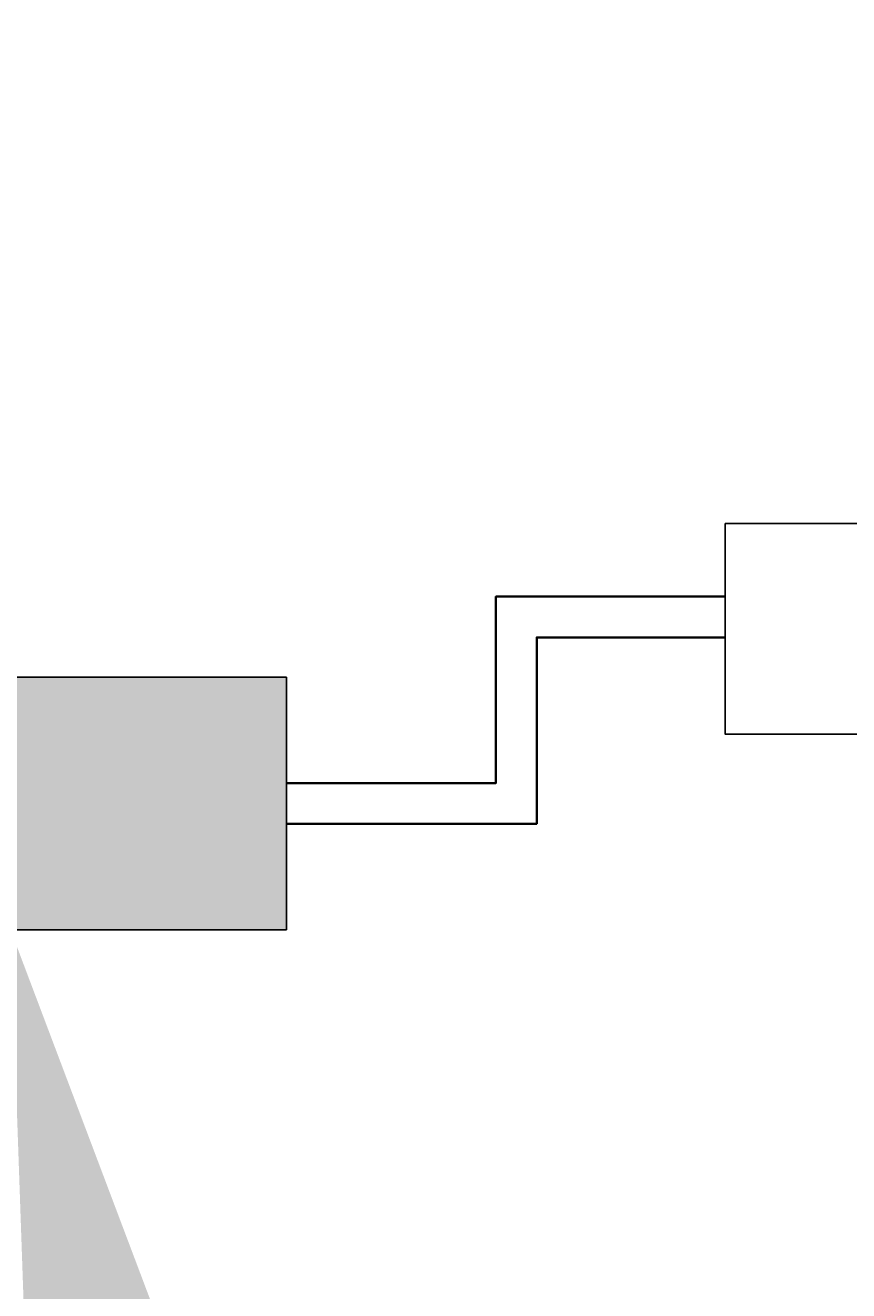
# Model space of a CAD drawing. Units: millimetres. Extents: x -22994 to 29398, y -19990 to 20176.
# Tile 14 of 135: x 58 to 79, y 21 to 52. Entities that reach past the tile are written whole.
import ezdxf
from ezdxf import colors
from ezdxf.entities.mleader import LeaderData, LeaderLine
from ezdxf.math import Vec2, Vec3

# ---------------------------------------------------------------- set-up
doc = ezdxf.new("R2010")
doc.units = ezdxf.units.MM
doc.header["$MEASUREMENT"] = 0
for name, color, linetype, lineweight in [('M-ANNO-TEXT', 7, 'Continuous', 25), ('M-DIMS', 2, 'Continuous', 18), ('M-EQPM', 7, 'Continuous', 25), ('M-EQPM-PATT', 7, 'Continuous', 18), ('M-PIPE', 7, 'Continuous', 35)]:
    doc.layers.add(name, color=color, linetype=linetype, lineweight=lineweight)
doc.styles.get("Standard").update_dxf_attribs({"font": 'arial.ttf'})
doc.dimstyles.get("Standard").update_dxf_attribs({"dimtxt": 0.18, "dimasz": 10000, "dimexe": 0.18, "dimexo": 0.0625, "dimgap": 0.09, "dimtad": 0, "dimtih": 1, "dimtoh": 1, "dimdec": 0, "dimzin": 0, "dimdsep": 46, "dimtxsty": 'Standard', "dimcen": 0.09, "dimadec": 0, "dimazin": 0, "dimtfac": 1, "dimtdec": 0, "dimtofl": 0, "dimtmove": 0, "dimatfit": 3, "dimfxl": 1, "dimtolj": 1, "dimtzin": 0, "dimlwd": 30, "dimarcsym": 0})

# ---------------------------------------------------------------- blocks, each defined once
blk = doc.blocks.new('*D2')
at = {"layer": 'Defpoints', "color": 0, "transparency": 16777216}
for p in [(6.677, 10.271), (290.852, 10.271), (290.852, -5.079)]:
    blk.add_point(p, dxfattribs=at)
at = {"layer": 'M-DIMS', "color": 0, "lineweight": -2, "transparency": 16777216}
for p, q in [((6.677, 10.209), (6.677, -5.259)), ((290.852, 10.209), (290.852, -5.259))]:
    blk.add_line(p, q, dxfattribs=at)
at = {"layer": 'M-DIMS', "color": 0, "lineweight": 30, "transparency": 16777216}
for p, q in [((-9993.323, -5.079), (-19993.323, -5.079)), ((10290.852, -5.079), (20290.852, -5.079))]:
    blk.add_line(p, q, dxfattribs=at)
at = {"layer": 'M-DIMS', "color": 0, "transparency": 16777216}
for points in [[(-9993.323, 1661.588), (-9993.323, -1671.745), (6.677, -5.079)], [(10290.852, 1661.588), (10290.852, -1671.745), (290.852, -5.079)]]:
    blk.add_solid(points, dxfattribs=at)
at = {"layer": 'M-DIMS', "color": 0, "transparency": 16777216, "insert": (148.765, -5.079), "char_height": 0.18, "attachment_point": 5}
blk.add_mtext('\\A1;284.2', dxfattribs=at)
blk = doc.blocks.new('*D3')
at = {"layer": 'Defpoints', "color": 0, "transparency": 16777216}
for p in [(110.265, 204.165), (110.265, 176.366), (95.833, 127.967)]:
    blk.add_point(p, dxfattribs=at)
at = {"layer": 'M-DIMS', "color": 0, "lineweight": 30, "transparency": 16777216}
for p, q in [((-9904.167, 204.165), (-19904.167, 204.165)), ((10110.265, 204.165), (20110.265, 204.165))]:
    blk.add_line(p, q, dxfattribs=at)
at = {"layer": 'M-DIMS', "color": 0, "lineweight": -2, "transparency": 16777216}
for p, q in [((95.833, 128.03), (95.833, 204.345)), ((110.265, 176.429), (110.265, 204.345))]:
    blk.add_line(p, q, dxfattribs=at)
at = {"layer": 'M-DIMS', "color": 0, "transparency": 16777216}
for points in [[(-9904.167, 1870.832), (-9904.167, -1462.501), (95.833, 204.165)], [(10110.265, 1870.832), (10110.265, -1462.501), (110.265, 204.165)]]:
    blk.add_solid(points, dxfattribs=at)
at = {"layer": 'M-DIMS', "color": 0, "transparency": 16777216, "insert": (103.049, 204.165), "char_height": 0.18, "attachment_point": 5}
blk.add_mtext('\\A1;14.432', dxfattribs=at)
blk = doc.blocks.new('*D4')
at = {"layer": 'Defpoints', "color": 0, "transparency": 16777216}
for p in [(116.265, 204.165), (110.265, 176.366), (116.265, 176.366)]:
    blk.add_point(p, dxfattribs=at)
at = {"layer": 'M-DIMS', "color": 0, "lineweight": 30, "transparency": 16777216}
for p, q in [((-9889.735, 204.165), (-19889.735, 204.165)), ((10116.265, 204.165), (20116.265, 204.165))]:
    blk.add_line(p, q, dxfattribs=at)
at = {"layer": 'M-DIMS', "color": 0, "lineweight": -2, "transparency": 16777216}
for p, q in [((110.265, 176.429), (110.265, 204.345)), ((116.265, 176.429), (116.265, 204.345))]:
    blk.add_line(p, q, dxfattribs=at)
at = {"layer": 'M-DIMS', "color": 0, "transparency": 16777216}
for points in [[(-9889.735, 1870.832), (-9889.735, -1462.501), (110.265, 204.165)], [(10116.265, 1870.832), (10116.265, -1462.501), (116.265, 204.165)]]:
    blk.add_solid(points, dxfattribs=at)
at = {"layer": 'M-DIMS', "color": 0, "transparency": 16777216, "insert": (113.265, 204.165), "char_height": 0.18, "attachment_point": 5}
blk.add_mtext('\\A1;6', dxfattribs=at)
blk = doc.blocks.new('*D5')
at = {"layer": 'Defpoints', "color": 0, "transparency": 16777216}
for p in [(181.265, 204.165), (116.265, 176.366), (181.265, 176.366)]:
    blk.add_point(p, dxfattribs=at)
at = {"layer": 'M-DIMS', "color": 0, "lineweight": 30, "transparency": 16777216}
for p, q in [((-9883.735, 204.165), (-19883.735, 204.165)), ((10181.265, 204.165), (20181.265, 204.165))]:
    blk.add_line(p, q, dxfattribs=at)
at = {"layer": 'M-DIMS', "color": 0, "lineweight": -2, "transparency": 16777216}
for p, q in [((116.265, 176.429), (116.265, 204.345)), ((181.265, 176.429), (181.265, 204.345))]:
    blk.add_line(p, q, dxfattribs=at)
at = {"layer": 'M-DIMS', "color": 0, "transparency": 16777216}
for points in [[(-9883.735, 1870.832), (-9883.735, -1462.501), (116.265, 204.165)], [(10181.265, 1870.832), (10181.265, -1462.501), (181.265, 204.165)]]:
    blk.add_solid(points, dxfattribs=at)
at = {"layer": 'M-DIMS', "color": 0, "transparency": 16777216, "insert": (148.765, 204.165), "char_height": 0.18, "attachment_point": 5}
blk.add_mtext('\\A1;65', dxfattribs=at)
blk = doc.blocks.new('*D6')
at = {"layer": 'Defpoints', "color": 0, "transparency": 16777216}
for p in [(187.265, 204.165), (181.265, 176.366), (187.265, 176.366)]:
    blk.add_point(p, dxfattribs=at)
at = {"layer": 'M-DIMS', "color": 0, "lineweight": 30, "transparency": 16777216}
for p, q in [((-9818.735, 204.165), (-19818.735, 204.165)), ((10187.265, 204.165), (20187.265, 204.165))]:
    blk.add_line(p, q, dxfattribs=at)
at = {"layer": 'M-DIMS', "color": 0, "lineweight": -2, "transparency": 16777216}
for p, q in [((181.265, 176.429), (181.265, 204.345)), ((187.265, 176.429), (187.265, 204.345))]:
    blk.add_line(p, q, dxfattribs=at)
at = {"layer": 'M-DIMS', "color": 0, "transparency": 16777216}
for points in [[(-9818.735, 1870.832), (-9818.735, -1462.501), (181.265, 204.165)], [(10187.265, 1870.832), (10187.265, -1462.501), (187.265, 204.165)]]:
    blk.add_solid(points, dxfattribs=at)
at = {"layer": 'M-DIMS', "color": 0, "transparency": 16777216, "insert": (184.265, 204.165), "char_height": 0.18, "attachment_point": 5}
blk.add_mtext('\\A1;6', dxfattribs=at)
blk = doc.blocks.new('*D7')
at = {"layer": 'Defpoints', "color": 0, "transparency": 16777216}
for p in [(201.697, 204.165), (187.265, 176.366), (201.697, 127.967)]:
    blk.add_point(p, dxfattribs=at)
at = {"layer": 'M-DIMS', "color": 0, "lineweight": 30, "transparency": 16777216}
for p, q in [((-9812.735, 204.165), (-19812.735, 204.165)), ((10201.697, 204.165), (20201.697, 204.165))]:
    blk.add_line(p, q, dxfattribs=at)
at = {"layer": 'M-DIMS', "color": 0, "lineweight": -2, "transparency": 16777216}
for p, q in [((187.265, 176.429), (187.265, 204.345)), ((201.697, 128.03), (201.697, 204.345))]:
    blk.add_line(p, q, dxfattribs=at)
at = {"layer": 'M-DIMS', "color": 0, "transparency": 16777216}
for points in [[(-9812.735, 1870.832), (-9812.735, -1462.501), (187.265, 204.165)], [(10201.697, 1870.832), (10201.697, -1462.501), (201.697, 204.165)]]:
    blk.add_solid(points, dxfattribs=at)
at = {"layer": 'M-DIMS', "color": 0, "transparency": 16777216, "insert": (194.481, 204.165), "char_height": 0.18, "attachment_point": 5}
blk.add_mtext('\\A1;14.432', dxfattribs=at)
blk = doc.blocks.new('*D8')
at = {"layer": 'Defpoints', "color": 0, "transparency": 16777216}
for p in [(227.648, 204.165), (227.648, 146.73), (201.697, 127.967)]:
    blk.add_point(p, dxfattribs=at)
at = {"layer": 'M-DIMS', "color": 0, "lineweight": 30, "transparency": 16777216}
for p, q in [((-9798.303, 204.165), (-19798.303, 204.165)), ((10227.648, 204.165), (20227.648, 204.165))]:
    blk.add_line(p, q, dxfattribs=at)
at = {"layer": 'M-DIMS', "color": 0, "lineweight": -2, "transparency": 16777216}
for p, q in [((201.697, 128.03), (201.697, 204.345)), ((227.648, 146.792), (227.648, 204.345))]:
    blk.add_line(p, q, dxfattribs=at)
at = {"layer": 'M-DIMS', "color": 0, "transparency": 16777216}
for points in [[(-9798.303, 1870.832), (-9798.303, -1462.501), (201.697, 204.165)], [(10227.648, 1870.832), (10227.648, -1462.501), (227.648, 204.165)]]:
    blk.add_solid(points, dxfattribs=at)
at = {"layer": 'M-DIMS', "color": 0, "transparency": 16777216, "insert": (214.673, 204.165), "char_height": 0.18, "attachment_point": 5}
blk.add_mtext('\\A1;25.95', dxfattribs=at)
blk = doc.blocks.new('*D9')
at = {"layer": 'Defpoints', "color": 0, "transparency": 16777216}
for p in [(187.265, 176.366), (306.202, 176.366), (290.852, 10.271)]:
    blk.add_point(p, dxfattribs=at)
at = {"layer": 'M-DIMS', "color": 0, "lineweight": 30, "transparency": 16777216}
for p, q in [((306.202, 10176.366), (306.202, 20176.366)), ((306.202, -9989.729), (306.202, -19989.729))]:
    blk.add_line(p, q, dxfattribs=at)
at = {"layer": 'M-DIMS', "color": 0, "lineweight": -2, "transparency": 16777216}
for p, q in [((187.327, 176.366), (306.382, 176.366)), ((290.915, 10.271), (306.382, 10.271))]:
    blk.add_line(p, q, dxfattribs=at)
at = {"layer": 'M-DIMS', "color": 0, "transparency": 16777216}
for points in [[(-1360.465, 10176.366), (1972.869, 10176.366), (306.202, 176.366)], [(-1360.465, -9989.729), (1972.869, -9989.729), (306.202, 10.271)]]:
    blk.add_solid(points, dxfattribs=at)
at = {"layer": 'M-DIMS', "color": 0, "transparency": 16777216, "insert": (306.202, 93.319), "char_height": 0.18, "attachment_point": 5}
blk.add_mtext('\\A1;166.1', dxfattribs=at)
blk = doc.blocks.new('*D10')
at = {"layer": 'Defpoints', "color": 0, "transparency": 16777216}
for p in [(125.65, 136.071), (133.346, 136.071), (133.346, -5.079)]:
    blk.add_point(p, dxfattribs=at)
at = {"layer": 'M-DIMS', "color": 0, "lineweight": -2, "transparency": 16777216}
for p, q in [((125.65, 136.009), (125.65, -5.259)), ((133.346, 136.009), (133.346, -5.259))]:
    blk.add_line(p, q, dxfattribs=at)
at = {"layer": 'M-DIMS', "color": 0, "lineweight": 30, "transparency": 16777216}
for p, q in [((-9874.35, -5.079), (-19874.35, -5.079)), ((10133.346, -5.079), (20133.346, -5.079))]:
    blk.add_line(p, q, dxfattribs=at)
at = {"layer": 'M-DIMS', "color": 0, "transparency": 16777216}
for points in [[(-9874.35, 1661.588), (-9874.35, -1671.745), (125.65, -5.079)], [(10133.346, 1661.588), (10133.346, -1671.745), (133.346, -5.079)]]:
    blk.add_solid(points, dxfattribs=at)
at = {"layer": 'M-DIMS', "color": 0, "transparency": 16777216, "insert": (129.498, -5.079), "char_height": 0.18, "attachment_point": 5}
blk.add_mtext('\\A1;7.696', dxfattribs=at)
blk = doc.blocks.new('*D11')
at = {"layer": 'Defpoints', "color": 0, "transparency": 16777216}
for p in [(133.346, 136.071), (135.65, 136.071), (135.65, -5.079)]:
    blk.add_point(p, dxfattribs=at)
at = {"layer": 'M-DIMS', "color": 0, "lineweight": -2, "transparency": 16777216}
for p, q in [((133.346, 136.009), (133.346, -5.259)), ((135.65, 136.009), (135.65, -5.259))]:
    blk.add_line(p, q, dxfattribs=at)
at = {"layer": 'M-DIMS', "color": 0, "lineweight": 30, "transparency": 16777216}
for p, q in [((-9866.654, -5.079), (-19866.654, -5.079)), ((10135.65, -5.079), (20135.65, -5.079))]:
    blk.add_line(p, q, dxfattribs=at)
at = {"layer": 'M-DIMS', "color": 0, "transparency": 16777216}
for points in [[(-9866.654, 1661.588), (-9866.654, -1671.745), (133.346, -5.079)], [(10135.65, 1661.588), (10135.65, -1671.745), (135.65, -5.079)]]:
    blk.add_solid(points, dxfattribs=at)
at = {"layer": 'M-DIMS', "color": 0, "transparency": 16777216, "insert": (134.498, -5.079), "char_height": 0.18, "attachment_point": 5}
blk.add_mtext('\\A1;2.304', dxfattribs=at)
blk = doc.blocks.new('*D12')
at = {"layer": 'Defpoints', "color": 0, "transparency": 16777216}
for p in [(135.65, 136.071), (145.65, 136.071), (145.65, -5.079)]:
    blk.add_point(p, dxfattribs=at)
at = {"layer": 'M-DIMS', "color": 0, "lineweight": -2, "transparency": 16777216}
for p, q in [((135.65, 136.009), (135.65, -5.259)), ((145.65, 136.009), (145.65, -5.259))]:
    blk.add_line(p, q, dxfattribs=at)
at = {"layer": 'M-DIMS', "color": 0, "lineweight": 30, "transparency": 16777216}
for p, q in [((-9864.35, -5.079), (-19864.35, -5.079)), ((10145.65, -5.079), (20145.65, -5.079))]:
    blk.add_line(p, q, dxfattribs=at)
at = {"layer": 'M-DIMS', "color": 0, "transparency": 16777216}
for points in [[(-9864.35, 1661.588), (-9864.35, -1671.745), (135.65, -5.079)], [(10145.65, 1661.588), (10145.65, -1671.745), (145.65, -5.079)]]:
    blk.add_solid(points, dxfattribs=at)
at = {"layer": 'M-DIMS', "color": 0, "transparency": 16777216, "insert": (140.65, -5.079), "char_height": 0.18, "attachment_point": 5}
blk.add_mtext('\\A1;10', dxfattribs=at)
blk = doc.blocks.new('*D13')
at = {"layer": 'Defpoints', "color": 0, "transparency": 16777216}
for p in [(145.65, 136.071), (155.65, 136.071), (155.65, -5.079)]:
    blk.add_point(p, dxfattribs=at)
at = {"layer": 'M-DIMS', "color": 0, "lineweight": -2, "transparency": 16777216}
for p, q in [((145.65, 136.009), (145.65, -5.259)), ((155.65, 136.009), (155.65, -5.259))]:
    blk.add_line(p, q, dxfattribs=at)
at = {"layer": 'M-DIMS', "color": 0, "lineweight": 30, "transparency": 16777216}
for p, q in [((-9854.35, -5.079), (-19854.35, -5.079)), ((10155.65, -5.079), (20155.65, -5.079))]:
    blk.add_line(p, q, dxfattribs=at)
at = {"layer": 'M-DIMS', "color": 0, "transparency": 16777216}
for points in [[(-9854.35, 1661.588), (-9854.35, -1671.745), (145.65, -5.079)], [(10155.65, 1661.588), (10155.65, -1671.745), (155.65, -5.079)]]:
    blk.add_solid(points, dxfattribs=at)
at = {"layer": 'M-DIMS', "color": 0, "transparency": 16777216, "insert": (150.65, -5.079), "char_height": 0.18, "attachment_point": 5}
blk.add_mtext('\\A1;10', dxfattribs=at)
blk = doc.blocks.new('*D14')
at = {"layer": 'Defpoints', "color": 0, "transparency": 16777216}
for p in [(155.65, 136.071), (165.65, 136.071), (165.65, -5.079)]:
    blk.add_point(p, dxfattribs=at)
at = {"layer": 'M-DIMS', "color": 0, "lineweight": -2, "transparency": 16777216}
for p, q in [((155.65, 136.009), (155.65, -5.259)), ((165.65, 136.009), (165.65, -5.259))]:
    blk.add_line(p, q, dxfattribs=at)
at = {"layer": 'M-DIMS', "color": 0, "lineweight": 30, "transparency": 16777216}
for p, q in [((-9844.35, -5.079), (-19844.35, -5.079)), ((10165.65, -5.079), (20165.65, -5.079))]:
    blk.add_line(p, q, dxfattribs=at)
at = {"layer": 'M-DIMS', "color": 0, "transparency": 16777216}
for points in [[(-9844.35, 1661.588), (-9844.35, -1671.745), (155.65, -5.079)], [(10165.65, 1661.588), (10165.65, -1671.745), (165.65, -5.079)]]:
    blk.add_solid(points, dxfattribs=at)
at = {"layer": 'M-DIMS', "color": 0, "transparency": 16777216, "insert": (160.65, -5.079), "char_height": 0.18, "attachment_point": 5}
blk.add_mtext('\\A1;10', dxfattribs=at)
blk = doc.blocks.new('*D15')
at = {"layer": 'Defpoints', "color": 0, "transparency": 16777216}
for p in [(173.346, 154.788), (173.346, 136.071), (306.202, 136.071)]:
    blk.add_point(p, dxfattribs=at)
at = {"layer": 'M-DIMS', "color": 0, "lineweight": 30, "transparency": 16777216}
for p, q in [((306.202, 10154.788), (306.202, 20154.788)), ((306.202, -9863.929), (306.202, -19863.929))]:
    blk.add_line(p, q, dxfattribs=at)
at = {"layer": 'M-DIMS', "color": 0, "lineweight": -2, "transparency": 16777216}
for p, q in [((173.408, 154.788), (306.382, 154.788)), ((173.408, 136.071), (306.382, 136.071))]:
    blk.add_line(p, q, dxfattribs=at)
at = {"layer": 'M-DIMS', "color": 0, "transparency": 16777216}
for points in [[(-1360.465, 10154.788), (1972.869, 10154.788), (306.202, 154.788)], [(-1360.465, -9863.929), (1972.869, -9863.929), (306.202, 136.071)]]:
    blk.add_solid(points, dxfattribs=at)
at = {"layer": 'M-DIMS', "color": 0, "transparency": 16777216, "insert": (306.202, 145.43), "char_height": 0.18, "attachment_point": 5}
blk.add_mtext('\\A1;18.717', dxfattribs=at)
blk = doc.blocks.new('*D16')
at = {"layer": 'Defpoints', "color": 0, "transparency": 16777216}
for p in [(120.17, 204.165), (110.466, 48.035), (120.17, 48.035)]:
    blk.add_point(p, dxfattribs=at)
at = {"layer": 'M-DIMS', "color": 0, "lineweight": 30, "transparency": 16777216}
for p, q in [((-9889.534, 204.165), (-19889.534, 204.165)), ((10120.17, 204.165), (20120.17, 204.165))]:
    blk.add_line(p, q, dxfattribs=at)
at = {"layer": 'M-DIMS', "color": 0, "lineweight": -2, "transparency": 16777216}
for p, q in [((110.466, 48.097), (110.466, 204.345)), ((120.17, 48.097), (120.17, 204.345))]:
    blk.add_line(p, q, dxfattribs=at)
at = {"layer": 'M-DIMS', "color": 0, "transparency": 16777216}
for points in [[(-9889.534, 1870.832), (-9889.534, -1462.501), (110.466, 204.165)], [(10120.17, 1870.832), (10120.17, -1462.501), (120.17, 204.165)]]:
    blk.add_solid(points, dxfattribs=at)
at = {"layer": 'M-DIMS', "color": 0, "transparency": 16777216, "insert": (115.318, 204.165), "char_height": 0.18, "attachment_point": 5}
blk.add_mtext('\\A1;9.704', dxfattribs=at)
blk = doc.blocks.new('*D17')
at = {"layer": 'Defpoints', "color": 0, "transparency": 16777216}
for p in [(126.17, 204.165), (120.17, 48.035), (126.17, 48.035)]:
    blk.add_point(p, dxfattribs=at)
at = {"layer": 'M-DIMS', "color": 0, "lineweight": 30, "transparency": 16777216}
for p, q in [((-9879.83, 204.165), (-19879.83, 204.165)), ((10126.17, 204.165), (20126.17, 204.165))]:
    blk.add_line(p, q, dxfattribs=at)
at = {"layer": 'M-DIMS', "color": 0, "lineweight": -2, "transparency": 16777216}
for p, q in [((120.17, 48.097), (120.17, 204.345)), ((126.17, 48.097), (126.17, 204.345))]:
    blk.add_line(p, q, dxfattribs=at)
at = {"layer": 'M-DIMS', "color": 0, "transparency": 16777216}
for points in [[(-9879.83, 1870.832), (-9879.83, -1462.501), (120.17, 204.165)], [(10126.17, 1870.832), (10126.17, -1462.501), (126.17, 204.165)]]:
    blk.add_solid(points, dxfattribs=at)
at = {"layer": 'M-DIMS', "color": 0, "transparency": 16777216, "insert": (123.17, 204.165), "char_height": 0.18, "attachment_point": 5}
blk.add_mtext('\\A1;6', dxfattribs=at)
blk = doc.blocks.new('*D18')
at = {"layer": 'Defpoints', "color": 0, "transparency": 16777216}
for p in [(132.17, 204.165), (126.17, 48.035), (132.17, 48.035)]:
    blk.add_point(p, dxfattribs=at)
at = {"layer": 'M-DIMS', "color": 0, "lineweight": 30, "transparency": 16777216}
for p, q in [((-9873.83, 204.165), (-19873.83, 204.165)), ((10132.17, 204.165), (20132.17, 204.165))]:
    blk.add_line(p, q, dxfattribs=at)
at = {"layer": 'M-DIMS', "color": 0, "lineweight": -2, "transparency": 16777216}
for p, q in [((126.17, 48.097), (126.17, 204.345)), ((132.17, 48.097), (132.17, 204.345))]:
    blk.add_line(p, q, dxfattribs=at)
at = {"layer": 'M-DIMS', "color": 0, "transparency": 16777216}
for points in [[(-9873.83, 1870.832), (-9873.83, -1462.501), (126.17, 204.165)], [(10132.17, 1870.832), (10132.17, -1462.501), (132.17, 204.165)]]:
    blk.add_solid(points, dxfattribs=at)
at = {"layer": 'M-DIMS', "color": 0, "transparency": 16777216, "insert": (129.17, 204.165), "char_height": 0.18, "attachment_point": 5}
blk.add_mtext('\\A1;6', dxfattribs=at)
blk = doc.blocks.new('*D19')
at = {"layer": 'Defpoints', "color": 0, "transparency": 16777216}
for p in [(138.17, 204.165), (132.17, 48.035), (138.17, 48.035)]:
    blk.add_point(p, dxfattribs=at)
at = {"layer": 'M-DIMS', "color": 0, "lineweight": 30, "transparency": 16777216}
for p, q in [((-9867.83, 204.165), (-19867.83, 204.165)), ((10138.17, 204.165), (20138.17, 204.165))]:
    blk.add_line(p, q, dxfattribs=at)
at = {"layer": 'M-DIMS', "color": 0, "lineweight": -2, "transparency": 16777216}
for p, q in [((132.17, 48.097), (132.17, 204.345)), ((138.17, 48.097), (138.17, 204.345))]:
    blk.add_line(p, q, dxfattribs=at)
at = {"layer": 'M-DIMS', "color": 0, "transparency": 16777216}
for points in [[(-9867.83, 1870.832), (-9867.83, -1462.501), (132.17, 204.165)], [(10138.17, 1870.832), (10138.17, -1462.501), (138.17, 204.165)]]:
    blk.add_solid(points, dxfattribs=at)
at = {"layer": 'M-DIMS', "color": 0, "transparency": 16777216, "insert": (135.17, 204.165), "char_height": 0.18, "attachment_point": 5}
blk.add_mtext('\\A1;6', dxfattribs=at)
blk = doc.blocks.new('*D20')
at = {"layer": 'Defpoints', "color": 0, "transparency": 16777216}
for p in [(144.17, 204.165), (138.17, 48.035), (144.17, 48.035)]:
    blk.add_point(p, dxfattribs=at)
at = {"layer": 'M-DIMS', "color": 0, "lineweight": 30, "transparency": 16777216}
for p, q in [((-9861.83, 204.165), (-19861.83, 204.165)), ((10144.17, 204.165), (20144.17, 204.165))]:
    blk.add_line(p, q, dxfattribs=at)
at = {"layer": 'M-DIMS', "color": 0, "lineweight": -2, "transparency": 16777216}
for p, q in [((138.17, 48.097), (138.17, 204.345)), ((144.17, 48.097), (144.17, 204.345))]:
    blk.add_line(p, q, dxfattribs=at)
at = {"layer": 'M-DIMS', "color": 0, "transparency": 16777216}
for points in [[(-9861.83, 1870.832), (-9861.83, -1462.501), (138.17, 204.165)], [(10144.17, 1870.832), (10144.17, -1462.501), (144.17, 204.165)]]:
    blk.add_solid(points, dxfattribs=at)
at = {"layer": 'M-DIMS', "color": 0, "transparency": 16777216, "insert": (141.17, 204.165), "char_height": 0.18, "attachment_point": 5}
blk.add_mtext('\\A1;6', dxfattribs=at)
blk = doc.blocks.new('*D21')
at = {"layer": 'Defpoints', "color": 0, "transparency": 16777216}
for p in [(149.116, 204.165), (144.17, 48.035), (149.116, 48.035)]:
    blk.add_point(p, dxfattribs=at)
at = {"layer": 'M-DIMS', "color": 0, "lineweight": 30, "transparency": 16777216}
for p, q in [((-9855.83, 204.165), (-19855.83, 204.165)), ((10149.116, 204.165), (20149.116, 204.165))]:
    blk.add_line(p, q, dxfattribs=at)
at = {"layer": 'M-DIMS', "color": 0, "lineweight": -2, "transparency": 16777216}
for p, q in [((144.17, 48.097), (144.17, 204.345)), ((149.116, 48.097), (149.116, 204.345))]:
    blk.add_line(p, q, dxfattribs=at)
at = {"layer": 'M-DIMS', "color": 0, "transparency": 16777216}
for points in [[(-9855.83, 1870.832), (-9855.83, -1462.501), (144.17, 204.165)], [(10149.116, 1870.832), (10149.116, -1462.501), (149.116, 204.165)]]:
    blk.add_solid(points, dxfattribs=at)
at = {"layer": 'M-DIMS', "color": 0, "transparency": 16777216, "insert": (146.643, 204.165), "char_height": 0.18, "attachment_point": 5}
blk.add_mtext('\\A1;4.945', dxfattribs=at)
blk = doc.blocks.new('*D22')
at = {"layer": 'Defpoints', "color": 0, "transparency": 16777216}
for p in [(149.116, 30.99), (155.116, 30.99), (155.116, -5.079)]:
    blk.add_point(p, dxfattribs=at)
at = {"layer": 'M-DIMS', "color": 0, "lineweight": -2, "transparency": 16777216}
for p, q in [((149.116, 30.927), (149.116, -5.259)), ((155.116, 30.927), (155.116, -5.259))]:
    blk.add_line(p, q, dxfattribs=at)
at = {"layer": 'M-DIMS', "color": 0, "lineweight": 30, "transparency": 16777216}
for p, q in [((-9850.884, -5.079), (-19850.884, -5.079)), ((10155.116, -5.079), (20155.116, -5.079))]:
    blk.add_line(p, q, dxfattribs=at)
at = {"layer": 'M-DIMS', "color": 0, "transparency": 16777216}
for points in [[(-9850.884, 1661.588), (-9850.884, -1671.745), (149.116, -5.079)], [(10155.116, 1661.588), (10155.116, -1671.745), (155.116, -5.079)]]:
    blk.add_solid(points, dxfattribs=at)
at = {"layer": 'M-DIMS', "color": 0, "transparency": 16777216, "insert": (152.116, -5.079), "char_height": 0.18, "attachment_point": 5}
blk.add_mtext('\\A1;6', dxfattribs=at)
blk = doc.blocks.new('*D23')
at = {"layer": 'Defpoints', "color": 0, "transparency": 16777216}
for p in [(155.116, 30.99), (161.116, 30.99), (161.116, -5.079)]:
    blk.add_point(p, dxfattribs=at)
at = {"layer": 'M-DIMS', "color": 0, "lineweight": -2, "transparency": 16777216}
for p, q in [((155.116, 30.927), (155.116, -5.259)), ((161.116, 30.927), (161.116, -5.259))]:
    blk.add_line(p, q, dxfattribs=at)
at = {"layer": 'M-DIMS', "color": 0, "lineweight": 30, "transparency": 16777216}
for p, q in [((-9844.884, -5.079), (-19844.884, -5.079)), ((10161.116, -5.079), (20161.116, -5.079))]:
    blk.add_line(p, q, dxfattribs=at)
at = {"layer": 'M-DIMS', "color": 0, "transparency": 16777216}
for points in [[(-9844.884, 1661.588), (-9844.884, -1671.745), (155.116, -5.079)], [(10161.116, 1661.588), (10161.116, -1671.745), (161.116, -5.079)]]:
    blk.add_solid(points, dxfattribs=at)
at = {"layer": 'M-DIMS', "color": 0, "transparency": 16777216, "insert": (158.116, -5.079), "char_height": 0.18, "attachment_point": 5}
blk.add_mtext('\\A1;6', dxfattribs=at)
blk = doc.blocks.new('*D24')
at = {"layer": 'Defpoints', "color": 0, "transparency": 16777216}
for p in [(161.116, 30.99), (166.439, 30.99), (166.439, -5.079)]:
    blk.add_point(p, dxfattribs=at)
at = {"layer": 'M-DIMS', "color": 0, "lineweight": -2, "transparency": 16777216}
for p, q in [((161.116, 30.927), (161.116, -5.259)), ((166.439, 30.927), (166.439, -5.259))]:
    blk.add_line(p, q, dxfattribs=at)
at = {"layer": 'M-DIMS', "color": 0, "lineweight": 30, "transparency": 16777216}
for p, q in [((-9838.884, -5.079), (-19838.884, -5.079)), ((10166.439, -5.079), (20166.439, -5.079))]:
    blk.add_line(p, q, dxfattribs=at)
at = {"layer": 'M-DIMS', "color": 0, "transparency": 16777216}
for points in [[(-9838.884, 1661.588), (-9838.884, -1671.745), (161.116, -5.079)], [(10166.439, 1661.588), (10166.439, -1671.745), (166.439, -5.079)]]:
    blk.add_solid(points, dxfattribs=at)
at = {"layer": 'M-DIMS', "color": 0, "transparency": 16777216, "insert": (163.777, -5.079), "char_height": 0.18, "attachment_point": 5}
blk.add_mtext('\\A1;5.323', dxfattribs=at)
blk = doc.blocks.new('*D25')
at = {"layer": 'Defpoints', "color": 0, "transparency": 16777216}
for p in [(166.439, 30.99), (172.439, 30.99), (172.439, -5.079)]:
    blk.add_point(p, dxfattribs=at)
at = {"layer": 'M-DIMS', "color": 0, "lineweight": -2, "transparency": 16777216}
for p, q in [((166.439, 30.927), (166.439, -5.259)), ((172.439, 30.927), (172.439, -5.259))]:
    blk.add_line(p, q, dxfattribs=at)
at = {"layer": 'M-DIMS', "color": 0, "lineweight": 30, "transparency": 16777216}
for p, q in [((-9833.561, -5.079), (-19833.561, -5.079)), ((10172.439, -5.079), (20172.439, -5.079))]:
    blk.add_line(p, q, dxfattribs=at)
at = {"layer": 'M-DIMS', "color": 0, "transparency": 16777216}
for points in [[(-9833.561, 1661.588), (-9833.561, -1671.745), (166.439, -5.079)], [(10172.439, 1661.588), (10172.439, -1671.745), (172.439, -5.079)]]:
    blk.add_solid(points, dxfattribs=at)
at = {"layer": 'M-DIMS', "color": 0, "transparency": 16777216, "insert": (169.439, -5.079), "char_height": 0.18, "attachment_point": 5}
blk.add_mtext('\\A1;6', dxfattribs=at)
blk = doc.blocks.new('*D26')
at = {"layer": 'Defpoints', "color": 0, "transparency": 16777216}
for p in [(172.439, 30.99), (178.439, 30.99), (178.439, -5.079)]:
    blk.add_point(p, dxfattribs=at)
at = {"layer": 'M-DIMS', "color": 0, "lineweight": -2, "transparency": 16777216}
for p, q in [((172.439, 30.927), (172.439, -5.259)), ((178.439, 30.927), (178.439, -5.259))]:
    blk.add_line(p, q, dxfattribs=at)
at = {"layer": 'M-DIMS', "color": 0, "lineweight": 30, "transparency": 16777216}
for p, q in [((-9827.561, -5.079), (-19827.561, -5.079)), ((10178.439, -5.079), (20178.439, -5.079))]:
    blk.add_line(p, q, dxfattribs=at)
at = {"layer": 'M-DIMS', "color": 0, "transparency": 16777216}
for points in [[(-9827.561, 1661.588), (-9827.561, -1671.745), (172.439, -5.079)], [(10178.439, 1661.588), (10178.439, -1671.745), (178.439, -5.079)]]:
    blk.add_solid(points, dxfattribs=at)
at = {"layer": 'M-DIMS', "color": 0, "transparency": 16777216, "insert": (175.439, -5.079), "char_height": 0.18, "attachment_point": 5}
blk.add_mtext('\\A1;6', dxfattribs=at)
blk = doc.blocks.new('*D27')
at = {"layer": 'Defpoints', "color": 0, "transparency": 16777216}
for p in [(178.439, 30.99), (188.117, 30.99), (188.117, -5.079)]:
    blk.add_point(p, dxfattribs=at)
at = {"layer": 'M-DIMS', "color": 0, "lineweight": -2, "transparency": 16777216}
for p, q in [((178.439, 30.927), (178.439, -5.259)), ((188.117, 30.927), (188.117, -5.259))]:
    blk.add_line(p, q, dxfattribs=at)
at = {"layer": 'M-DIMS', "color": 0, "lineweight": 30, "transparency": 16777216}
for p, q in [((-9821.561, -5.079), (-19821.561, -5.079)), ((10188.117, -5.079), (20188.117, -5.079))]:
    blk.add_line(p, q, dxfattribs=at)
at = {"layer": 'M-DIMS', "color": 0, "transparency": 16777216}
for points in [[(-9821.561, 1661.588), (-9821.561, -1671.745), (178.439, -5.079)], [(10188.117, 1661.588), (10188.117, -1671.745), (188.117, -5.079)]]:
    blk.add_solid(points, dxfattribs=at)
at = {"layer": 'M-DIMS', "color": 0, "transparency": 16777216, "insert": (183.278, -5.079), "char_height": 0.18, "attachment_point": 5}
blk.add_mtext('\\A1;9.679', dxfattribs=at)
blk = doc.blocks.new('*D28')
at = {"layer": 'Defpoints', "color": 0, "transparency": 16777216}
for p in [(188.117, 48.035), (306.202, 48.035), (188.117, 30.99)]:
    blk.add_point(p, dxfattribs=at)
at = {"layer": 'M-DIMS', "color": 0, "lineweight": 30, "transparency": 16777216}
for p, q in [((306.202, 10048.035), (306.202, 20048.035)), ((306.202, -9969.01), (306.202, -19969.01))]:
    blk.add_line(p, q, dxfattribs=at)
at = {"layer": 'M-DIMS', "color": 0, "lineweight": -2, "transparency": 16777216}
for p, q in [((188.18, 48.035), (306.382, 48.035)), ((188.18, 30.99), (306.382, 30.99))]:
    blk.add_line(p, q, dxfattribs=at)
at = {"layer": 'M-DIMS', "color": 0, "transparency": 16777216}
for points in [[(-1360.465, 10048.035), (1972.869, 10048.035), (306.202, 48.035)], [(-1360.465, -9969.01), (1972.869, -9969.01), (306.202, 30.99)]]:
    blk.add_solid(points, dxfattribs=at)
at = {"layer": 'M-DIMS', "color": 0, "transparency": 16777216, "insert": (306.202, 39.512), "char_height": 0.18, "attachment_point": 5}
blk.add_mtext('\\A1;17.045', dxfattribs=at)
blk = doc.blocks.new('*D29')
at = {"layer": 'Defpoints', "color": 0, "transparency": 16777216}
for p in [(36.801, 80.045), (64.03, 80.045)]:
    blk.add_point(p, dxfattribs=at)
at = {"layer": 'M-DIMS', "color": 0, "lineweight": -2, "transparency": 16777216}
for p, q in [((50.325, 80.045), (50.505, 80.045)), ((50.415, 79.955), (50.415, 80.135))]:
    blk.add_line(p, q, dxfattribs=at)
at = {"layer": 'M-DIMS', "color": 0, "lineweight": 30, "transparency": 16777216}
blk.add_line((20064.03, 80.03), (10064.03, 80.038), dxfattribs=at)
at = {"layer": 'M-DIMS', "color": 0, "transparency": 16777216}
blk.add_solid([(10064.031, 1746.704), (10064.028, -1586.629), (64.03, 80.045)], dxfattribs=at)
at = {"layer": 'M-DIMS', "color": 0, "transparency": 16777216, "insert": (20064.521, 80.03), "char_height": 0.18, "attachment_point": 5}
blk.add_mtext('\\A1;∅27.23', dxfattribs=at)
blk = doc.blocks.new('*D36')
at = {"layer": 'Defpoints', "color": 0, "transparency": 16777216}
for p in [(46.39, 31.303), (46.387, 26.593)]:
    blk.add_point(p, dxfattribs=at)
at = {"layer": 'M-DIMS', "color": 0, "lineweight": 30, "transparency": 16777216}
for p, q in [((57.15, 20031.301), (51.77, 10031.302)), ((10057.15, 20031.301), (57.15, 20031.301))]:
    blk.add_line(p, q, dxfattribs=at)
at = {"layer": 'M-DIMS', "color": 0, "lineweight": -2, "transparency": 16777216}
for p, q in [((46.299, 28.948), (46.479, 28.948)), ((46.389, 28.858), (46.389, 29.038))]:
    blk.add_line(p, q, dxfattribs=at)
at = {"layer": 'M-DIMS', "color": 0, "transparency": 16777216}
blk.add_solid([(-1614.896, 10032.199), (1718.436, 10030.405), (46.39, 31.303)], dxfattribs=at)
at = {"layer": 'M-DIMS', "color": 0, "transparency": 16777216, "insert": (10057.554, 20031.301), "char_height": 0.18, "attachment_point": 5}
blk.add_mtext('\\A1;∅4.71', dxfattribs=at)
blk = doc.blocks.new('*D37')
at = {"layer": 'Defpoints', "color": 0, "transparency": 16777216}
for p in [(54.834, 118.615), (59.494, 118.614)]:
    blk.add_point(p, dxfattribs=at)
at = {"layer": 'M-DIMS', "color": 0, "lineweight": -2, "transparency": 16777216}
for p, q in [((57.074, 118.614), (57.254, 118.614)), ((57.164, 118.524), (57.164, 118.704))]:
    blk.add_line(p, q, dxfattribs=at)
at = {"layer": 'M-DIMS', "color": 0, "lineweight": 30, "transparency": 16777216}
blk.add_line((20059.493, 116.253), (10059.494, 117.434), dxfattribs=at)
at = {"layer": 'M-DIMS', "color": 0, "transparency": 16777216}
blk.add_solid([(10059.69, 1784.1), (10059.297, -1549.233), (59.494, 118.614)], dxfattribs=at)
at = {"layer": 'M-DIMS', "color": 0, "transparency": 16777216, "insert": (20059.985, 116.253), "char_height": 0.18, "attachment_point": 5}
blk.add_mtext('\\A1;∅4.659', dxfattribs=at)

msp = doc.modelspace()

# ---------------------------------------------------------------- hatches: boundary and pattern name
at = {"layer": 'M-EQPM-PATT'}
h = msp.add_hatch(color=256, dxfattribs=at)
h.set_gradient(color1=(242, 103, 34), color2=(242, 103, 34), tint=1, name='CYLINDER')
h.paths.add_polyline_path([(53.5912, 30.0354), (64.8905, 30.0354), (64.8905, 36.2325), (46.3887, 36.2325, 2.6954641)])
h.paths.add_polyline_path([(44.0337, 28.9485, -1), (48.7438, 28.9485, -1)], flags=16)
h.paths.add_polyline_path([(75.6657, 119.7012), (75.6657, 125.8983), (57.1639, 125.8983, 2.6954641), (64.3664, 119.7012)])
h.paths.add_polyline_path([(59.4936, 118.6143, -1), (54.8343, 118.6143, -1)], flags=16)

# ---------------------------------------------------------------- linework, layer by layer
at = {"layer": 'M-EQPM'}
for p, q in [((46.3887, 36.2325), (64.8905, 36.2325)), ((64.8905, 36.2325), (64.8905, 30.0354)), ((64.8905, 30.0354), (53.5912, 30.0354))]:
    msp.add_line(p, q, dxfattribs=at)
msp.add_lwpolyline([(75.6375, 39.9986), (88.0111, 39.9986), (88.0111, 34.8308), (75.6375, 34.8308)], close=True, dxfattribs=at)
at = {"layer": 'M-PIPE'}
for points in [[(64.8905, 33.6339), (70.0182, 33.6339), (70.0182, 38.2029), (75.6375, 38.2029)], [(64.8905, 32.6339), (71.0182, 32.6339), (71.0182, 37.2029), (75.6375, 37.2029)]]:
    msp.add_lwpolyline(points, dxfattribs=at)

# ---------------------------------------------------------------- dimensions: what is measured, and where the dimension line sits
at = {"layer": 'M-DIMS'}
for base, p1, p2, override, picture, middle in [((306.202, 176.3662), (290.852, 10.2713), (187.2647, 176.3662), {"dimdec": 1, "dimlfac": 1, "dimrnd": 0, "dimzin": 0, "dimdsep": 46, "dimlunit": 2}, '*D9', (306.202, 93.3187)), ((306.202, 136.0713), (173.3459, 154.788), (173.3459, 136.0713), {"dimdec": 3, "dimlfac": 1, "dimrnd": 0, "dimzin": 0, "dimdsep": 46, "dimlunit": 2}, '*D15', (306.202, 145.4297)), ((306.202, 48.0349), (188.1175, 30.9895), (188.1175, 48.0349), {"dimdec": 3, "dimlfac": 1, "dimrnd": 0, "dimzin": 0, "dimdsep": 46, "dimlunit": 2}, '*D28', (306.202, 39.5122))]:
    dim = msp.add_linear_dim(base=base, p1=p1, p2=p2, angle=90, dimstyle='Standard', override=override, dxfattribs=at)
    dim.commit()
    dim.dimension.update_dxf_attribs({"geometry": picture, "text_midpoint": middle})
dim = msp.add_diameter_dim_2p(p1=(46.3875, 26.5934), p2=(46.39, 31.3035), dimstyle='Standard', override={"dimdec": 2, "dimlfac": 1, "dimrnd": 0, "dimzin": 0, "dimdsep": 46, "dimlunit": 2}, dxfattribs=at)
dim.commit()
dim.dimension.update_dxf_attribs({"geometry": '*D36', "text_midpoint": (10057.5542, 20031.3006), "dimtype": 163})
for base, p1, p2, override, picture, middle in [((110.2647, 204.1654), (95.8327, 127.967), (110.2647, 176.3662), {"dimdec": 3, "dimlfac": 1, "dimrnd": 0, "dimzin": 0, "dimdsep": 46, "dimlunit": 2}, '*D3', (103.0487, 204.1654)), ((116.2647, 204.1654), (110.2647, 176.3662), (116.2647, 176.3662), {"dimdec": 0, "dimlfac": 1, "dimrnd": 0, "dimzin": 0, "dimdsep": 46, "dimlunit": 2}, '*D4', (113.2647, 204.1654)), ((120.1702, 204.1654), (110.4658, 48.0349), (120.1702, 48.0349), {"dimdec": 3, "dimlfac": 1, "dimrnd": 0, "dimzin": 0, "dimdsep": 46, "dimlunit": 2}, '*D16', (115.318, 204.1654)), ((181.2647, 204.1654), (116.2647, 176.3662), (181.2647, 176.3662), {"dimdec": 0, "dimlfac": 1, "dimrnd": 0, "dimzin": 0, "dimdsep": 46, "dimlunit": 2}, '*D5', (148.7647, 204.1654)), ((126.1702, 204.1654), (120.1702, 48.0349), (126.1702, 48.0349), {"dimdec": 0, "dimlfac": 1, "dimrnd": 0, "dimzin": 0, "dimdsep": 46, "dimlunit": 2}, '*D17', (123.1702, 204.1654)), ((132.1702, 204.1654), (126.1702, 48.0349), (132.1702, 48.0349), {"dimdec": 0, "dimlfac": 1, "dimrnd": 0, "dimzin": 0, "dimdsep": 46, "dimlunit": 2}, '*D18', (129.1702, 204.1654)), ((138.1702, 204.1654), (132.1702, 48.0349), (138.1702, 48.0349), {"dimdec": 0, "dimlfac": 1, "dimrnd": 0, "dimzin": 0, "dimdsep": 46, "dimlunit": 2}, '*D19', (135.1702, 204.1654)), ((144.1702, 204.1654), (138.1702, 48.0349), (144.1702, 48.0349), {"dimdec": 0, "dimlfac": 1, "dimrnd": 0, "dimzin": 0, "dimdsep": 46, "dimlunit": 2}, '*D20', (141.1702, 204.1654)), ((149.11567, 204.16539), (144.17023, 48.03494), (149.11567, 48.03494), {"dimdec": 3, "dimlfac": 1, "dimrnd": 0, "dimzin": 0, "dimdsep": 46, "dimlunit": 2}, '*D21', (146.64295, 204.16539)), ((187.2647, 204.1654), (181.2647, 176.3662), (187.2647, 176.3662), {"dimdec": 0, "dimlfac": 1, "dimrnd": 0, "dimzin": 0, "dimdsep": 46, "dimlunit": 2}, '*D6', (184.2647, 204.1654)), ((201.6967, 204.1654), (187.2647, 176.3662), (201.6967, 127.967), {"dimdec": 3, "dimlfac": 1, "dimrnd": 0, "dimzin": 0, "dimdsep": 46, "dimlunit": 2}, '*D7', (194.4807, 204.1654)), ((227.6485, 204.1654), (201.6967, 127.967), (227.6485, 146.7296), {"dimdec": 2, "dimlfac": 1, "dimrnd": 0, "dimzin": 0, "dimdsep": 46, "dimlunit": 2}, '*D8', (214.6726, 204.1654)), ((290.852, -5.0787), (6.6773, 10.2713), (290.852, 10.2713), {"dimdec": 1, "dimlfac": 1, "dimrnd": 0, "dimzin": 0, "dimdsep": 46, "dimlunit": 2}, '*D2', (148.7647, -5.0787)), ((133.3459, -5.0787), (125.6498, 136.0713), (133.3459, 136.0713), {"dimdec": 3, "dimlfac": 1, "dimrnd": 0, "dimzin": 0, "dimdsep": 46, "dimlunit": 2}, '*D10', (129.4978, -5.0787)), ((135.6498, -5.0787), (133.3459, 136.0713), (135.6498, 136.0713), {"dimdec": 3, "dimlfac": 1, "dimrnd": 0, "dimzin": 0, "dimdsep": 46, "dimlunit": 2}, '*D11', (134.4978, -5.0787)), ((145.6498, -5.0787), (135.6498, 136.0713), (145.6498, 136.0713), {"dimdec": 0, "dimlfac": 1, "dimrnd": 0, "dimzin": 0, "dimdsep": 46, "dimlunit": 2}, '*D12', (140.6498, -5.0787)), ((155.6498, -5.0787), (145.6498, 136.0713), (155.6498, 136.0713), {"dimdec": 0, "dimlfac": 1, "dimrnd": 0, "dimzin": 0, "dimdsep": 46, "dimlunit": 2}, '*D13', (150.6498, -5.0787)), ((155.1157, -5.0787), (149.1157, 30.9895), (155.1157, 30.9895), {"dimdec": 0, "dimlfac": 1, "dimrnd": 0, "dimzin": 0, "dimdsep": 46, "dimlunit": 2}, '*D22', (152.1157, -5.0787)), ((161.1157, -5.0787), (155.1157, 30.9895), (161.1157, 30.9895), {"dimdec": 0, "dimlfac": 1, "dimrnd": 0, "dimzin": 0, "dimdsep": 46, "dimlunit": 2}, '*D23', (158.1157, -5.0787)), ((165.6498, -5.0787), (155.6498, 136.0713), (165.6498, 136.0713), {"dimdec": 0, "dimlfac": 1, "dimrnd": 0, "dimzin": 0, "dimdsep": 46, "dimlunit": 2}, '*D14', (160.6498, -5.0787)), ((166.4387, -5.0787), (161.1157, 30.9895), (166.4387, 30.9895), {"dimdec": 3, "dimlfac": 1, "dimrnd": 0, "dimzin": 0, "dimdsep": 46, "dimlunit": 2}, '*D24', (163.7772, -5.0787)), ((172.4387, -5.0787), (166.4387, 30.9895), (172.4387, 30.9895), {"dimdec": 0, "dimlfac": 1, "dimrnd": 0, "dimzin": 0, "dimdsep": 46, "dimlunit": 2}, '*D25', (169.4387, -5.0787)), ((178.4387, -5.0787), (172.4387, 30.9895), (178.4387, 30.9895), {"dimdec": 0, "dimlfac": 1, "dimrnd": 0, "dimzin": 0, "dimdsep": 46, "dimlunit": 2}, '*D26', (175.4387, -5.0787)), ((188.1175, -5.0787), (178.4387, 30.9895), (188.1175, 30.9895), {"dimdec": 3, "dimlfac": 1, "dimrnd": 0, "dimzin": 0, "dimdsep": 46, "dimlunit": 2}, '*D27', (183.2781, -5.0787))]:
    dim = msp.add_linear_dim(base=base, p1=p1, p2=p2, dimstyle='Standard', override=override, dxfattribs=at)
    dim.commit()
    dim.dimension.update_dxf_attribs({"geometry": picture, "text_midpoint": middle})
for p1, p2, override, picture, middle in [((54.8343, 118.6145), (59.4936, 118.614), {"dimdec": 3, "dimlfac": 1, "dimrnd": 0, "dimzin": 0, "dimdsep": 46, "dimlunit": 2}, '*D37', (20059.4934, 116.2531)), ((36.8006, 80.045), (64.0296, 80.045), {"dimdec": 2, "dimlfac": 1, "dimrnd": 0, "dimzin": 0, "dimdsep": 46, "dimlunit": 2}, '*D29', (20064.0296, 80.0303))]:
    dim = msp.add_diameter_dim_2p(p1=p1, p2=p2, dimstyle='Standard', override=override, dxfattribs=at)
    dim.commit()
    dim.dimension.update_dxf_attribs({"geometry": picture, "text_midpoint": middle})

# ---------------------------------------------------------------- leaders
at = {"layer": 'M-ANNO-TEXT'}
ml = msp.add_multileader_mtext('Standard', dxfattribs=at)
ml.set_content('Distributing heater', color=256)
ml.set_leader_properties()
ml.build(insert=Vec2(0, 0))
ml.multileader.update_dxf_attribs({"dogleg_length": 0.36, "arrow_head_size": 200})
ctx = ml.context
ctx.base_point, ctx.arrow_head_size, ctx.landing_gap_size, ctx.plane_origin = Vec3(86.8201, 4.9577), 200, 0.09, Vec3(80.3507, 34.8308)
notes = []
notes.append((ctx, [(1, (1, 1, 0), (82.8058, 4.9577), (1, 0), 4.0143, [(0, [(80.3507, 34.8308)], 0, [])])]))
ctx.mtext.insert, ctx.mtext.flow_direction = Vec3(86.9101, 7.5457), 5
ml = msp.add_multileader_mtext('Standard', dxfattribs=at)
ml.set_content('Circulating pump', color=256)
ml.set_leader_properties()
ml.build(insert=Vec2(0, 0))
ml.multileader.update_dxf_attribs({"dogleg_length": 0.36, "arrow_head_size": 200})
ctx = ml.context
ctx.base_point, ctx.arrow_head_size, ctx.landing_gap_size, ctx.plane_origin = Vec3(13.008, 3.5951), 200, 0.09, Vec3(56.3887, 19.3615)
ctx.text_align_type = 2
notes.append((ctx, [(1, (1, 1, 0), (63.4296, 3.5951), (-1, 0), 8.8146, [(0, [(58.1278, 30.0354)], 0, [])])]))
ctx.mtext.insert, ctx.mtext.alignment, ctx.mtext.flow_direction = Vec3(54.525, 6.1831), 3, 5
for ctx, leaders in notes:
    for number, flags, end, landing, length, lines in leaders:
        leader = LeaderData()
        leader.index, (leader.has_last_leader_line, leader.has_dogleg_vector, leader.attachment_direction) = number, flags
        leader.last_leader_point, leader.dogleg_vector, leader.dogleg_length = Vec3(end), Vec3(landing), length
        for number, points, colour, breaks in lines:
            line = LeaderLine()
            line.index, line.vertices, line.color, line.breaks = number, Vec3.list(points), colors.encode_raw_color(colour), breaks
            leader.lines.append(line)
        ctx.leaders.append(leader)

doc.saveas('drawing.dxf')
